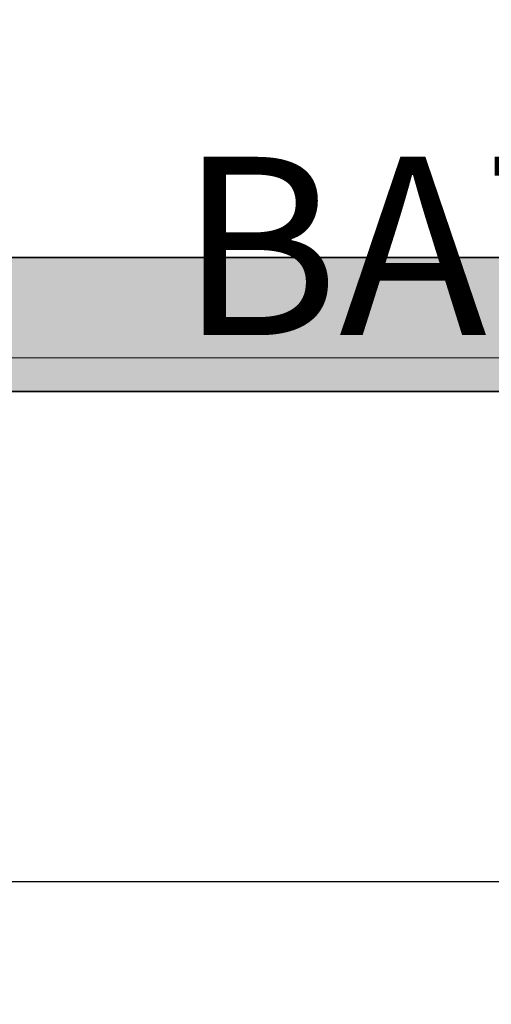
# Model space of a CAD drawing. Units: inches. Extents: x 2696 to 3240, y 1564 to 2310.
# Tile 48 of 76: x 2786 to 2802, y 2071 to 2104. Entities that reach past the tile are written whole.
import ezdxf

# ---------------------------------------------------------------- set-up
doc = ezdxf.new("R2010")
doc.units = ezdxf.units.IN
for name, color, linetype, lineweight in [('A-ANNO-DIMS', 3, 'Continuous', 18), ('A-WALL', 7, 'Continuous', 35), ('A-WALL-PATT', 9, 'Continuous', 13)]:
    doc.layers.add(name, color=color, linetype=linetype, lineweight=lineweight)
doc.styles.add('TIMES NEW', font='times.ttf')
doc.dimstyles.new('Siddhuu', dxfattribs={"dimtxt": 6, "dimasz": 2.5, "dimexe": 1.25, "dimexo": 0.625, "dimtad": 1, "dimdec": 1, "dimlunit": 4, "dimtxsty": 'TIMES NEW', "dimcen": 2.5, "dimclrd": 256, "dimclre": 1, "dimclrt": 7, "dimadec": 0, "dimazin": 0, "dimtfac": 1, "dimtdec": 1, "dimtmove": 0, "dimatfit": 3, "dimfxl": 1, "dimtolj": 1, "dimlwd": -1, "dimarcsym": 0})

# ---------------------------------------------------------------- blocks, each defined once
blk = doc.blocks.new('*D40')
at = {"layer": 'A-ANNO-DIMS', "color": 1, "lineweight": -2, "transparency": 16777216}
for p, q in [((2777.266, 2091.826), (2777.266, 2093.576)), ((2784.764, 2091.826), (2784.764, 2093.576))]:
    blk.add_line(p, q, dxfattribs=at)
at = {"layer": 'A-ANNO-DIMS', "transparency": 16777216}
for p, q in [((2779.766, 2092.326), (2782.264, 2092.326)), ((2784.764, 2092.326), (2902.458, 2092.326))]:
    blk.add_line(p, q, dxfattribs=at)
for points in [[(2779.766, 2092.742), (2779.766, 2091.909), (2777.266, 2092.326)], [(2782.264, 2092.742), (2782.264, 2091.909), (2784.764, 2092.326)]]:
    blk.add_solid(points, dxfattribs=at)
at = {"layer": 'Defpoints', "color": 0, "transparency": 16777216}
for p in [(2784.764, 2092.326), (2777.266, 2091.201), (2784.764, 2091.201)]:
    blk.add_point(p, dxfattribs=at)
at = {"layer": 'A-ANNO-DIMS', "color": 7, "transparency": 16777216, "insert": (2844.861, 2096.094), "char_height": 6, "attachment_point": 5, "style": 'TIMES NEW'}
blk.add_mtext('\\A1;BATH FITTING 0\'-7 1/2" TYP.', dxfattribs=at)
blk = doc.blocks.new('*D62')
at = {"layer": 'A-ANNO-DIMS', "color": 1, "lineweight": -2, "transparency": 16777216}
for p, q in [((2965.084, 2140.701), (2709.361, 2140.701)), ((2965.084, 2063.591), (2709.361, 2063.591))]:
    blk.add_line(p, q, dxfattribs=at)
at = {"layer": 'A-ANNO-DIMS', "transparency": 16777216}
blk.add_line((2710.611, 2066.091), (2710.611, 2138.201), dxfattribs=at)
for points in [[(2710.195, 2138.201), (2711.028, 2138.201), (2710.611, 2140.701)], [(2710.195, 2066.091), (2711.028, 2066.091), (2710.611, 2063.591)]]:
    blk.add_solid(points, dxfattribs=at)
at = {"layer": 'Defpoints', "color": 0, "transparency": 16777216}
for p in [(2710.611, 2140.701), (2965.709, 2140.701), (2965.709, 2063.591)]:
    blk.add_point(p, dxfattribs=at)
at = {"layer": 'A-ANNO-DIMS', "color": 7, "transparency": 16777216, "insert": (2706.934, 2102.146), "char_height": 6, "attachment_point": 5, "rotation": 90, "style": 'TIMES NEW'}
blk.add_mtext('\\A1;6\'-5"', dxfattribs=at)
blk = doc.blocks.new('*D64')
at = {"layer": 'A-ANNO-DIMS', "color": 1, "lineweight": -2, "transparency": 16777216}
for p, q in [((3073.084, 2206.701), (2709.361, 2206.701)), ((3068.584, 1989.201), (2709.361, 1989.201))]:
    blk.add_line(p, q, dxfattribs=at)
at = {"layer": 'A-ANNO-DIMS', "transparency": 16777216}
blk.add_line((2710.611, 1991.701), (2710.611, 2204.201), dxfattribs=at)
for points in [[(2710.195, 2204.201), (2711.028, 2204.201), (2710.611, 2206.701)], [(2710.195, 1991.701), (2711.028, 1991.701), (2710.611, 1989.201)]]:
    blk.add_solid(points, dxfattribs=at)
at = {"layer": 'Defpoints', "color": 0, "transparency": 16777216}
for p in [(2710.611, 2206.701), (3073.709, 2206.701), (3069.209, 1989.201)]:
    blk.add_point(p, dxfattribs=at)
at = {"layer": 'A-ANNO-DIMS', "color": 7, "transparency": 16777216, "insert": (2706.85, 2097.951), "char_height": 6, "attachment_point": 5, "rotation": 90, "style": 'TIMES NEW'}
blk.add_mtext('\\A1;18\'-1 1/2"', dxfattribs=at)
blk = doc.blocks.new('*D66')
at = {"layer": 'A-ANNO-DIMS', "color": 1, "lineweight": -2, "transparency": 16777216}
for p, q in [((3077.584, 2122.701), (2709.361, 2122.701)), ((3077.584, 2074.701), (2709.361, 2074.701))]:
    blk.add_line(p, q, dxfattribs=at)
at = {"layer": 'A-ANNO-DIMS', "transparency": 16777216}
blk.add_line((2710.611, 2077.201), (2710.611, 2120.201), dxfattribs=at)
for points in [[(2710.195, 2120.201), (2711.028, 2120.201), (2710.611, 2122.701)], [(2710.195, 2077.201), (2711.028, 2077.201), (2710.611, 2074.701)]]:
    blk.add_solid(points, dxfattribs=at)
at = {"layer": 'Defpoints', "color": 0, "transparency": 16777216}
for p in [(2710.611, 2122.701), (3078.209, 2122.701), (3078.209, 2074.701)]:
    blk.add_point(p, dxfattribs=at)
at = {"layer": 'A-ANNO-DIMS', "color": 7, "transparency": 16777216, "insert": (2706.934, 2098.701), "char_height": 6, "attachment_point": 5, "rotation": 90, "style": 'TIMES NEW'}
blk.add_mtext('\\A1;4\'-0"', dxfattribs=at)

msp = doc.modelspace()

# ---------------------------------------------------------------- hatches: boundary and pattern name
at = {"layer": 'A-WALL-PATT', "transparency": 33554556}
h = msp.add_hatch(color=256, dxfattribs=at)
h.dxf.hatch_style = 1
h.paths.add_polyline_path([(2879.111, 2253.201), (2905.91, 2253.201), (2905.91, 2262.201), (2841.889, 2262.201), (2841.889, 2253.201), (2870.111, 2253.201), (2870.111, 2176.601), (2965.709, 2176.601), (2965.709, 2206.701), (2973.583, 2206.701), (2973.583, 2215.701), (2965.709, 2215.701), (2965.709, 2262.201), (2929.91, 2262.201), (2929.91, 2253.201), (2956.709, 2253.201), (2956.709, 2185.601), (2879.111, 2185.601)])
h.paths.add_polyline_path([(2782.834, 2262.201), (2745.611, 2262.201), (2745.611, 2228.729), (2754.611, 2228.729), (2754.611, 2253.201), (2782.834, 2253.201)])
h.paths.add_polyline_path([(2754.611, 2136.201), (2965.709, 2136.201), (2965.709, 2145.201), (2879.111, 2145.201), (2879.111, 2147.074), (2877.34, 2147.074), (2870.111, 2147.074), (2870.111, 2145.201), (2754.611, 2145.201), (2754.611, 2169.674), (2745.611, 2169.674), (2745.611, 2000.201), (2754.611, 2000.201), (2754.611, 2019.201), (2849.083, 2019.201), (2849.083, 2023.701), (2841.209, 2023.701), (2841.209, 2051.827), (2836.709, 2051.827), (2836.709, 2023.701), (2754.611, 2023.701), (2754.611, 2091.201), (2836.709, 2091.201), (2836.709, 2087.827), (2841.209, 2087.827), (2841.209, 2095.701), (2754.611, 2095.701)])
h.paths.add_polyline_path([(2965.709, 2136.201), (2956.709, 2136.201), (2956.709, 2023.701), (2885.083, 2023.701), (2885.083, 2019.201), (2956.709, 2019.201), (2956.709, 1950.575), (2965.709, 1950.575), (2965.709, 1980.201), (2973.583, 1980.201), (2973.583, 1989.201), (2965.709, 1989.201)])
h.paths.add_polyline_path([(2754.611, 1906.701), (2880.209, 1906.701), (2884.709, 1906.701), (2956.709, 1906.701), (2956.709, 1792.701), (2944.709, 1792.701), (2944.709, 1783.701), (2956.709, 1783.701), (2956.709, 1740.201), (2884.709, 1740.201), (2884.709, 1783.701), (2896.709, 1783.701), (2896.709, 1792.701), (2884.709, 1792.701), (2884.709, 1846.701), (2880.209, 1846.701), (2880.209, 1740.201), (2754.611, 1740.201), (2754.611, 1777.201), (2745.611, 1777.201), (2745.611, 1692.701), (2754.611, 1692.701), (2754.611, 1731.201), (2956.709, 1731.201), (2956.709, 1723.327), (2965.709, 1723.327), (2965.709, 1884.201), (2973.583, 1884.201), (2973.583, 1893.201), (2965.709, 1893.201), (2965.709, 1914.575), (2956.709, 1914.575), (2956.709, 1911.201), (2754.611, 1911.201), (2754.611, 1930.201), (2745.611, 1930.201), (2745.611, 1817.201), (2754.611, 1817.201), (2754.611, 1854.201), (2826.611, 1854.201), (2826.611, 1868.827), (2822.111, 1868.827), (2822.111, 1858.701), (2754.611, 1858.701)])
h.paths.add_polyline_path([(2965.709, 1656.201), (3008.237, 1656.201), (3008.237, 1665.201), (2965.709, 1665.201), (2965.709, 1693.327), (2956.709, 1693.327), (2956.709, 1686.201), (2934.583, 1686.201), (2934.583, 1681.701), (2956.709, 1681.701), (2956.709, 1614.201), (2896.709, 1614.201), (2896.709, 1681.701), (2904.583, 1681.701), (2904.583, 1686.201), (2892.209, 1686.201), (2892.209, 1614.201), (2858.41, 1614.201), (2858.41, 1605.201), (2965.709, 1605.201)])
h.paths.add_polyline_path([(2788.41, 1614.201), (2754.611, 1614.201), (2754.611, 1652.701), (2745.611, 1652.701), (2745.611, 1605.201), (2788.41, 1605.201)])
h.paths.add_polyline_path([(3199.611, 1633.048), (3190.611, 1633.048), (3190.611, 1614.201), (3082.611, 1614.201), (3082.611, 1665.201), (3070.237, 1665.201), (3070.237, 1656.201), (3078.111, 1656.201), (3078.111, 1605.201), (3199.611, 1605.201)])
h.paths.add_polyline_path([(3199.611, 1702.048), (3190.611, 1702.048), (3190.611, 1699.701), (3106.611, 1699.701), (3106.611, 1747.701), (3190.611, 1747.701), (3190.611, 1752.201), (3082.611, 1752.201), (3082.611, 1760.075), (3078.111, 1760.075), (3078.111, 1747.701), (3102.111, 1747.701), (3102.111, 1699.701), (3078.111, 1699.701), (3078.111, 1695.201), (3190.611, 1695.201), (3190.611, 1676.355), (3199.611, 1676.355)])
h.paths.add_polyline_path([(3199.611, 1783.201), (3190.611, 1783.201), (3190.611, 1745.355), (3199.611, 1745.355)])
h.paths.add_polyline_path([(3082.611, 1884.201), (3190.611, 1884.201), (3190.611, 1853.201), (3199.611, 1853.201), (3199.611, 1901.701), (3190.611, 1901.701), (3190.611, 1893.201), (3005.583, 1893.201), (3005.583, 1891.281), (3005.583, 1884.201), (3078.111, 1884.201), (3078.111, 1792.075), (3082.611, 1792.075)])
h.paths.add_polyline_path([(3199.611, 1994.701), (3190.611, 1994.701), (3190.611, 1989.201), (3073.709, 1989.201), (3073.709, 2034.201), (3069.209, 2034.201), (3069.209, 1989.201), (3005.583, 1989.201), (3005.583, 1980.201), (3190.611, 1980.201), (3190.611, 1971.701), (3199.611, 1971.701)])
h.paths.add_polyline_path([(3199.611, 2155.201), (3190.611, 2155.201), (3190.611, 2064.701), (3199.611, 2064.701)])
h.paths.add_polyline_path([(3190.611, 2074.701), (3106.611, 2074.701), (3106.611, 2122.701), (3190.611, 2122.701), (3190.611, 2127.201), (3082.709, 2127.201), (3082.709, 2135.075), (3073.709, 2135.075), (3073.709, 2122.701), (3102.111, 2122.701), (3102.111, 2074.701), (3069.209, 2074.701), (3069.209, 2070.201), (3190.611, 2070.201)])
h.paths.add_polyline_path([(3082.709, 2253.201), (3190.611, 2253.201), (3190.611, 2225.201), (3199.611, 2225.201), (3199.611, 2262.201), (3073.709, 2262.201), (3073.709, 2215.701), (3035.583, 2215.701), (3035.583, 2206.701), (3073.709, 2206.701), (3073.709, 2171.075), (3082.709, 2171.075)])

# ---------------------------------------------------------------- linework, layer by layer
at = {"layer": 'A-WALL'}
for p, q in [((2754.611, 2095.701), (2841.209, 2095.701)), ((2754.611, 2091.201), (2836.709, 2091.201))]:
    msp.add_line(p, q, dxfattribs=at)

# ---------------------------------------------------------------- dimensions: what is measured, and where the dimension line sits
at = {"layer": 'A-ANNO-DIMS'}
for base, p1, p2, picture, middle in [((2710.611, 2206.701), (3069.209, 1989.201), (3073.709, 2206.701), '*D64', (2706.85, 2097.951)), ((2710.611, 2140.701), (2965.709, 2063.591), (2965.709, 2140.701), '*D62', (2706.934, 2102.146)), ((2710.611, 2122.701), (3078.209, 2074.701), (3078.209, 2122.701), '*D66', (2706.934, 2098.701))]:
    dim = msp.add_linear_dim(base=base, p1=p1, p2=p2, angle=90, dimstyle='Siddhuu', override={"dimdec": 1, "dimlfac": 1, "dimrnd": 0, "dimzin": 1, "dimdsep": 46, "dimlunit": 4, "dimfrac": 2}, dxfattribs=at)
    dim.commit()
    dim.dimension.update_dxf_attribs({"geometry": picture, "text_midpoint": middle})
dim = msp.add_linear_dim(base=(2784.764, 2092.326), p1=(2777.266, 2091.201), p2=(2784.764, 2091.201), text='BATH FITTING <> TYP.', dimstyle='Siddhuu', override={"dimdec": 1, "dimlfac": 1, "dimrnd": 0, "dimzin": 1, "dimdsep": 46, "dimlunit": 4, "dimfrac": 2}, dxfattribs=at)
dim.commit()
dim.dimension.update_dxf_attribs({"geometry": '*D40', "text_midpoint": (2844.861, 2096.094)})

doc.saveas('drawing.dxf')
